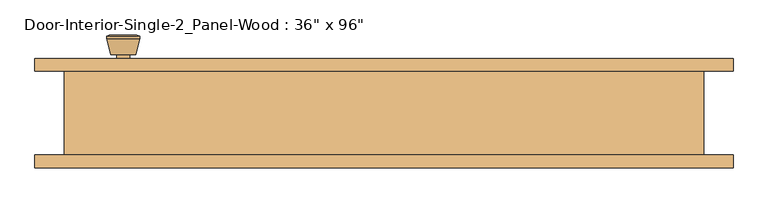
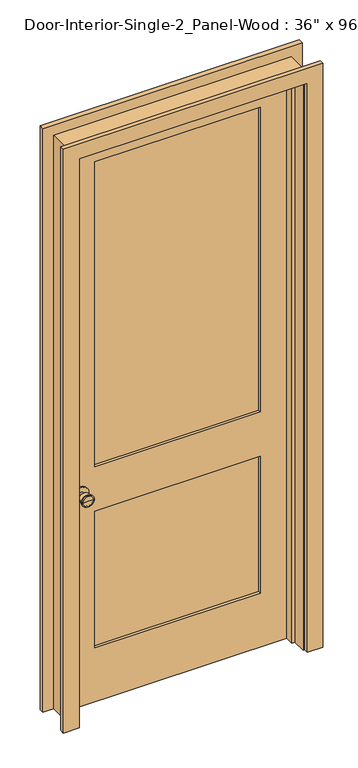
"""IFC4 building model written with IfcOpenShell, lengths in millimetres: door geometry."""

from ifc_helpers import new_model, si_unit, point, frame, frame_2d, origin, place, context, project, spatial, polyline, circle_curve, trimmed, segment, composite_curve, outline, extrude, faceted_brep, source, transform, mapped, element, save
from ifc_brep_helpers import plane_surface, cylinder_surface, revolved_surface, advanced_brep


def door_1a517266(model_context):
    return source(origin(), model_context, "Body", "SolidModel", [
        advanced_brep(
        [(-393.7, 19.4, 914.4), (-383.7, 19.4, 914.4), (-403.7, 19.4, 914.4), (-373.2241324, -29.6, 914.4), (-393.7, -29.6, 914.4), (-414.1758676, -29.6, 914.4), (-368.7, -27.7721319, 914.4), (-418.7, -27.7721319, 914.4), (-368.7, -24.3084537, 914.4), (-418.7, -24.3084537, 914.4), (-375.063764, 0.4, 914.4), (-412.336236, 0.4, 914.4), (-383.7, 0.4, 914.4), (-403.7, 0.4, 914.4)],
        [
            (0, 1),
            (1, 2, circle_curve(frame((-393.7, 19.4, 914.4), z_axis=(0.0, 1.0, 0.0), x_axis=(-1.0, 0.0, 0.0)), 10.0)),
            (2, 0),
            (2, 1, circle_curve(frame((-393.7, 19.4, 914.4), z_axis=(0.0, 1.0, 0.0), x_axis=(-1.0, 0.0, 0.0)), 10.0)),
            (3, 4),
            (4, 5),
            (5, 3, circle_curve(frame((-393.7, -29.6, 914.4), z_axis=(0.0, -1.0, 0.0), x_axis=(-1.0, 0.0, 0.0)), 20.4758676)),
            (3, 5, circle_curve(frame((-393.7, -29.6, 914.4), z_axis=(0.0, -1.0, 0.0), x_axis=(-1.0, 0.0, 0.0)), 20.4758676)),
            (6, 3),
            (5, 7),
            (7, 6, circle_curve(frame((-393.7, -27.7721319, 914.4), z_axis=(0.0, -1.0, 0.0), x_axis=(-1.0, 0.0, 0.0)), 25.0)),
            (6, 7, circle_curve(frame((-393.7, -27.7721319, 914.4), z_axis=(0.0, -1.0, 0.0), x_axis=(-1.0, 0.0, 0.0)), 25.0)),
            (8, 6),
            (7, 9),
            (9, 8, circle_curve(frame((-393.7, -24.3084537, 914.4), z_axis=(0.0, -1.0, 0.0), x_axis=(-1.0, 0.0, 0.0)), 25.0)),
            (8, 9, circle_curve(frame((-393.7, -24.3084537, 914.4), z_axis=(0.0, -1.0, 0.0), x_axis=(-1.0, 0.0, 0.0)), 25.0)),
            (10, 8),
            (9, 11),
            (11, 10, circle_curve(frame((-393.7, 0.4, 914.4), z_axis=(0.0, -1.0, 0.0), x_axis=(-1.0, 0.0, 0.0)), 18.636236)),
            (10, 11, circle_curve(frame((-393.7, 0.4, 914.4), z_axis=(0.0, -1.0, 0.0), x_axis=(-1.0, 0.0, 0.0)), 18.636236)),
            (12, 10),
            (11, 13),
            (13, 12, circle_curve(frame((-393.7, 0.4, 914.4), z_axis=(0.0, -1.0, 0.0), x_axis=(-1.0, 0.0, 0.0)), 10.0)),
            (12, 13, circle_curve(frame((-393.7, 0.4, 914.4), z_axis=(0.0, -1.0, 0.0), x_axis=(-1.0, 0.0, 0.0)), 10.0)),
            (1, 12),
            (13, 2),
        ],
        [
            plane_surface(frame((-393.7, 19.4, 914.4), z_axis=(0.0, 1.0, 0.0), x_axis=(-1.0, 0.0, 0.0))),
            plane_surface(frame((-393.7, -29.6, 914.4), z_axis=(0.0, -1.0, 0.0), x_axis=(-1.0, 0.0, 0.0))),
            revolved_surface(polyline([(-414.1758676, -29.6, 914.4), (-418.7, -27.7721319, 914.4)]), (-393.7, 19.4, 914.4), (0.0, 1.0, 0.0)),
            cylinder_surface(frame((-393.7, 19.4, 914.4), z_axis=(0.0, 1.0, 0.0), x_axis=(-1.0, 0.0, 0.0)), 25.0),
            revolved_surface(polyline([(-418.7, -24.3084537, 914.4), (-412.336236, 0.4, 914.4)]), (-393.7, 19.4, 914.4), (0.0, 1.0, 0.0)),
            plane_surface(frame((-393.7, 0.4, 914.4), z_axis=(0.0, 1.0, 0.0), x_axis=(-1.0, 0.0, 0.0))),
            cylinder_surface(frame((-393.7, 19.4, 914.4), z_axis=(0.0, 1.0, 0.0), x_axis=(-1.0, 0.0, 0.0)), 10.0),
        ],
        [
            (0, [[1, 2, 3]]),
            (0, [[-3, 4, -1]]),
            (1, [[5, 6, 7]]),
            (1, [[-6, -5, 8]]),
            (2, [[9, -7, 10, 11]]),
            (2, [[-10, -8, -9, 12]]),
            (3, [[13, -11, 14, 15]]),
            (3, [[-14, -12, -13, 16]]),
            (4, [[17, -15, 18, 19]]),
            (4, [[-18, -16, -17, 20]]),
            (5, [[21, -19, 22, 23]]),
            (5, [[-22, -20, -21, 24]]),
            (6, [[25, -23, 26, -2]]),
            (6, [[-26, -24, -25, -4]]),
        ],
    ),
        extrude(outline(composite_curve([segment(trimmed(circle_curve(frame_2d((914.4, -393.7)), 30.0), [point((914.4, -423.7))], [point((914.4, -363.7))], False, "CARTESIAN"), True, "CONTINUOUS"), segment(trimmed(circle_curve(frame_2d((914.4, -393.7)), 30.0), [point((914.4, -363.7))], [point((914.4, -423.7))], False, "CARTESIAN"), True, "CONTINUOUS")], self_intersect=False)), frame((0.0, 19.4, 0.0), z_axis=(0.0, 1.0, 0.0), x_axis=(0.0, 0.0, 1.0)), (0.0, 0.0, 1.0), 6.0),
        advanced_brep(
        [(-393.7, 66.325, 914.4), (-403.7, 66.325, 914.4), (-383.7, 66.325, 914.4), (-373.2241324, 115.325, 914.4), (-414.1758676, 115.325, 914.4), (-393.7, 115.325, 914.4), (-368.7, 113.4971319, 914.4), (-418.7, 113.4971319, 914.4), (-368.7, 110.0334537, 914.4), (-418.7, 110.0334537, 914.4), (-375.063764, 85.325, 914.4), (-412.336236, 85.325, 914.4), (-383.7, 85.325, 914.4), (-403.7, 85.325, 914.4)],
        [
            (0, 1),
            (1, 2, circle_curve(frame((-393.7, 66.325, 914.4), z_axis=(0.0, -1.0, 0.0), x_axis=(-1.0, 0.0, 0.0)), 10.0)),
            (2, 0),
            (2, 1, circle_curve(frame((-393.7, 66.325, 914.4), z_axis=(0.0, -1.0, 0.0), x_axis=(-1.0, 0.0, 0.0)), 10.0)),
            (3, 4, circle_curve(frame((-393.7, 115.325, 914.4), z_axis=(0.0, 1.0, 0.0), x_axis=(-1.0, 0.0, 0.0)), 20.4758676)),
            (4, 5),
            (5, 3),
            (4, 3, circle_curve(frame((-393.7, 115.325, 914.4), z_axis=(0.0, 1.0, 0.0), x_axis=(-1.0, 0.0, 0.0)), 20.4758676)),
            (6, 7, circle_curve(frame((-393.7, 113.4971319, 914.4), z_axis=(0.0, 1.0, 0.0), x_axis=(-1.0, 0.0, 0.0)), 25.0)),
            (7, 4),
            (3, 6),
            (7, 6, circle_curve(frame((-393.7, 113.4971319, 914.4), z_axis=(0.0, 1.0, 0.0), x_axis=(-1.0, 0.0, 0.0)), 25.0)),
            (8, 9, circle_curve(frame((-393.7, 110.0334537, 914.4), z_axis=(0.0, 1.0, 0.0), x_axis=(-1.0, 0.0, 0.0)), 25.0)),
            (9, 7),
            (6, 8),
            (9, 8, circle_curve(frame((-393.7, 110.0334537, 914.4), z_axis=(0.0, 1.0, 0.0), x_axis=(-1.0, 0.0, 0.0)), 25.0)),
            (10, 11, circle_curve(frame((-393.7, 85.325, 914.4), z_axis=(0.0, 1.0, 0.0), x_axis=(-1.0, 0.0, 0.0)), 18.636236)),
            (11, 9),
            (8, 10),
            (11, 10, circle_curve(frame((-393.7, 85.325, 914.4), z_axis=(0.0, 1.0, 0.0), x_axis=(-1.0, 0.0, 0.0)), 18.636236)),
            (12, 13, circle_curve(frame((-393.7, 85.325, 914.4), z_axis=(0.0, 1.0, 0.0), x_axis=(-1.0, 0.0, 0.0)), 10.0)),
            (13, 11),
            (10, 12),
            (13, 12, circle_curve(frame((-393.7, 85.325, 914.4), z_axis=(0.0, 1.0, 0.0), x_axis=(-1.0, 0.0, 0.0)), 10.0)),
            (1, 13),
            (12, 2),
        ],
        [
            plane_surface(frame((-393.7, 66.325, 914.4), z_axis=(0.0, -1.0, 0.0), x_axis=(-1.0, 0.0, 0.0))),
            plane_surface(frame((-393.7, 115.325, 914.4), z_axis=(0.0, 1.0, 0.0), x_axis=(-1.0, 0.0, 0.0))),
            revolved_surface(polyline([(-414.1758676, 115.325, 914.4), (-418.7, 113.4971319, 914.4)]), (-393.7, 66.325, 914.4), (0.0, -1.0, 0.0)),
            cylinder_surface(frame((-393.7, 66.325, 914.4), z_axis=(0.0, -1.0, 0.0), x_axis=(-1.0, 0.0, 0.0)), 25.0),
            revolved_surface(polyline([(-418.7, 110.0334537, 914.4), (-412.336236, 85.325, 914.4)]), (-393.7, 66.325, 914.4), (0.0, -1.0, 0.0)),
            plane_surface(frame((-393.7, 85.325, 914.4), z_axis=(0.0, -1.0, 0.0), x_axis=(-1.0, 0.0, 0.0))),
            cylinder_surface(frame((-393.7, 66.325, 914.4), z_axis=(0.0, -1.0, 0.0), x_axis=(-1.0, 0.0, 0.0)), 10.0),
        ],
        [
            (0, [[1, 2, 3]]),
            (0, [[-3, 4, -1]]),
            (1, [[5, 6, 7]]),
            (1, [[8, -7, -6]]),
            (2, [[9, 10, -5, 11]]),
            (2, [[12, -11, -8, -10]]),
            (3, [[13, 14, -9, 15]]),
            (3, [[16, -15, -12, -14]]),
            (4, [[17, 18, -13, 19]]),
            (4, [[20, -19, -16, -18]]),
            (5, [[21, 22, -17, 23]]),
            (5, [[24, -23, -20, -22]]),
            (6, [[-2, 25, -21, 26]]),
            (6, [[-4, -26, -24, -25]]),
        ],
    ),
        extrude(outline(composite_curve([segment(trimmed(circle_curve(frame_2d((914.4, -393.7)), 30.0), [point((914.4, -423.7))], [point((914.4, -363.7))], False, "CARTESIAN"), True, "CONTINUOUS"), segment(trimmed(circle_curve(frame_2d((914.4, -393.7)), 30.0), [point((914.4, -363.7))], [point((914.4, -423.7))], False, "CARTESIAN"), True, "CONTINUOUS")], self_intersect=False)), frame((0.0, 60.325, 0.0), z_axis=(0.0, 1.0, 0.0), x_axis=(0.0, 0.0, 1.0)), (0.0, 0.0, 1.0), 6.0),
        faceted_brep([(482.6, 60.325, 0.0), (482.6, -66.675, 0.0), (457.2, -66.675, 0.0), (457.2, -9.525, 0.0), (444.5, -9.525, 0.0), (444.5, 25.4, 0.0), (457.2, 25.4, 0.0), (457.2, 60.325, 0.0), (482.6, 60.325, 2463.8), (482.6, -66.675, 2463.8), (-482.6, -66.675, 2463.8), (-482.6, -66.675, 0.0), (-457.2, -66.675, 0.0), (-457.2, -66.675, 2438.4), (457.2, -66.675, 2438.4), (457.2, -9.525, 2438.4), (-457.2, -9.525, 2438.4), (-457.2, -9.525, 0.0), (-444.5, -9.525, 0.0), (-444.5, -9.525, 2425.7), (444.5, -9.525, 2425.7), (444.5, 25.4, 2425.7), (-444.5, 25.4, 2425.7), (-444.5, 25.4, 0.0), (-457.2, 25.4, 0.0), (-457.2, 25.4, 2438.4), (457.2, 25.4, 2438.4), (457.2, 60.325, 2438.4), (-457.2, 60.325, 2438.4), (-457.2, 60.325, 0.0), (-482.6, 60.325, 0.0), (-482.6, 60.325, 2463.8)], [[[0, 1, 2, 3, 4, 5, 6, 7]], [[1, 0, 8, 9]], [[2, 1, 9, 10, 11, 12, 13, 14]], [[3, 2, 14, 15]], [[4, 3, 15, 16, 17, 18, 19, 20]], [[5, 4, 20, 21]], [[6, 5, 21, 22, 23, 24, 25, 26]], [[7, 6, 26, 27]], [[0, 7, 27, 28, 29, 30, 31, 8]], [[9, 8, 31, 10]], [[15, 14, 13, 16]], [[21, 20, 19, 22]], [[27, 26, 25, 28]], [[30, 29, 24, 23, 18, 17, 12, 11]], [[10, 31, 30, 11]], [[16, 13, 12, 17]], [[22, 19, 18, 23]], [[28, 25, 24, 29]]]),
        extrude(outline(polyline([(2438.4, -457.2), (0.0, -457.2), (0.0, 457.2), (2438.4, 457.2), (2438.4, -457.2)]), holes=[polyline([(2319.3375, -336.55), (2319.3375, 336.55), (1009.65, 336.55), (1009.65, -336.55), (2319.3375, -336.55)]), polyline([(819.15, -336.55), (819.15, 336.55), (231.775, 336.55), (231.775, -336.55), (819.15, -336.55)])]), frame((0.0, 25.4, 0.0), z_axis=(0.0, 1.0, 0.0), x_axis=(0.0, 0.0, 1.0)), (0.0, 0.0, 1.0), 34.925),
        extrude(outline(polyline([(336.55, 37.0416667), (-336.55, 37.0416667), (-336.55, 48.6833333), (336.55, 48.6833333), (336.55, 37.0416667)])), frame((0.0, 0.0, 1009.65), z_axis=(0.0, 0.0, 1.0), x_axis=(1.0, 0.0, 0.0)), (0.0, 0.0, 1.0), 1309.6875),
        extrude(outline(polyline([(336.55, 37.0416667), (-336.55, 37.0416667), (-336.55, 48.6833333), (336.55, 48.6833333), (336.55, 37.0416667)])), frame((0.0, 0.0, 231.775), z_axis=(0.0, 0.0, 1.0), x_axis=(1.0, 0.0, 0.0)), (0.0, 0.0, 1.0), 587.375),
        extrude(outline(polyline([(0.0, 463.55), (0.0, 527.05), (2508.25, 527.05), (2508.25, -527.05), (0.0, -527.05), (0.0, -463.55), (2444.75, -463.55), (2444.75, 463.55), (0.0, 463.55)])), frame((0.0, 60.325, 0.0), z_axis=(0.0, 1.0, 0.0), x_axis=(0.0, 0.0, 1.0)), (0.0, 0.0, 1.0), 19.05),
        extrude(outline(polyline([(0.0, 463.55), (0.0, 527.05), (2508.25, 527.05), (2508.25, -527.05), (0.0, -527.05), (0.0, -463.55), (2444.75, -463.55), (2444.75, 463.55), (0.0, 463.55)])), frame((0.0, -85.725, 0.0), z_axis=(0.0, 1.0, 0.0), x_axis=(0.0, 0.0, 1.0)), (0.0, 0.0, 1.0), 19.05),
    ])


if __name__ == "__main__":
    model = new_model("IFC4")
    model_context = context("Model", 3, world=origin())
    ifc_project = project(units=[si_unit("LENGTHUNIT", "METRE", prefix="MILLI")], contexts=[model_context])
    site = spatial("IfcSite", under=ifc_project)
    building = spatial("IfcBuilding", under=site)
    placement = place(None, origin())
    door_shape = door_1a517266(model_context)
    element("IfcDoor", 1, ObjectType="Door-Interior-Single-2_Panel-Wood : 36\" x 96\"", at=placement, inside=building, context=model_context, shape_type="MappedRepresentation", body=[
        mapped(door_shape, transform((0.0, 0.0, 0.0), x_axis=(1.0, 0.0, 0.0), y_axis=(0.0, 1.0, 0.0), z_axis=(0.0, 0.0, 1.0))),
    ])
    save(model, "model.ifc")

# Revit data of these elements
# Type "Door-Interior-Single-2_Panel-Wood : 36\" x 96\""
#   Type Mark = "10"
#   Assembly Code = "C1020300"
#   Analytic Construction = "Wooden"
#   Top Rail = 0' - 4 11/16"
#   Thickness = 0' - 1 3/8"
#   Thermal Resistance (R) = 2.5876 (h·ft²·°F)/BTU
#   Swing Angle [instance default] = 90.00°
#   Stiles = 0' - 4 3/4"
#   Rough Width = 3' - 2"
#   Rough Height = 8' - 1"
#   Lock Rail = 0' - 7 1/2"
#   Height = 8' - 0"
#   Width = 3' - 0"
#   Heat Transfer Coefficient (U) = 0.3865 BTU/(h·ft²·°F)
#   Bottom Rail = 0' - 9 1/8"
#   Trim Material = Cherry
#   Panel Material = Cherry
#   Frame Material = Cherry
#   Door Handle Material = Aluminum
#   Visual Light Transmittance = 0
#   Solar Heat Gain Coefficient = 0
#   Wall Closure = (empty or 0)
#   Function = (empty or 0)
# Element 1 (IfcDoor, "Door-Interior-Single-2_Panel-Wood : 36\" x 96\"")
#   Materials on its faces: "Cherry", "Aluminum"
# Materials
#   "Cherry": class "Wood", colour RGB 226 177 128, transparency 0, Description = "Prunus Serotina", Cost = 0
#   "Aluminum": class "Metal", colour RGB 247 247 247, transparency 0, Description = "Aluminum 6061", Cost = 0
